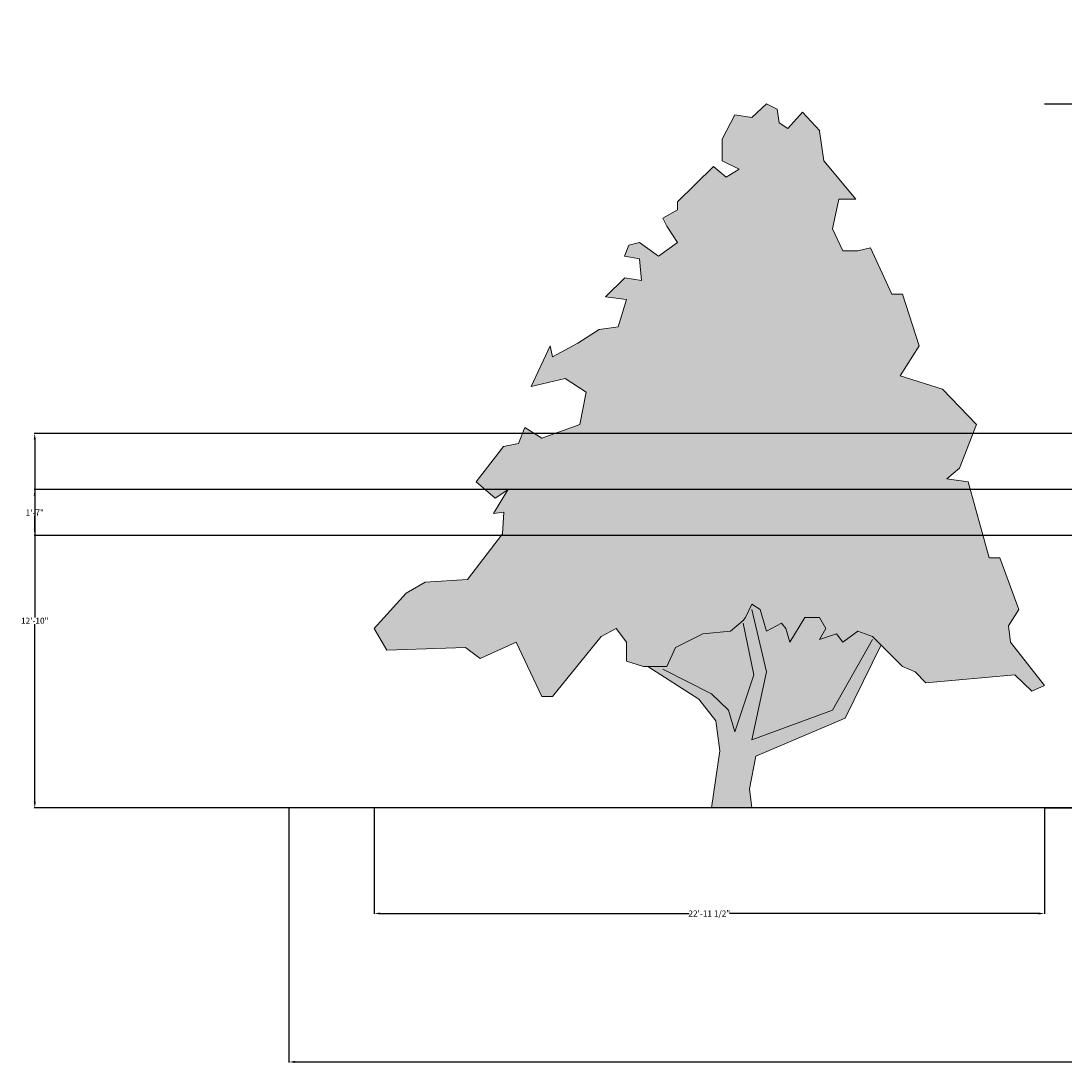
# Model space of a CAD drawing. Units: inches. Extents: x 481 to 2783, y 1975 to 3327.
# Tile 1 of 13: x 481 to 910, y 2015 to 2447. Entities that reach past the tile are written whole.
import ezdxf

# ---------------------------------------------------------------- set-up
doc = ezdxf.new("R2010")
doc.units = ezdxf.units.IN
doc.header["$MEASUREMENT"] = 0
for name, color, linetype, lineweight in [('A-ANNO-DIMS', 50, 'Continuous', 18), ('C-TOPO', 7, 'Continuous', 25), ('L-PLNT', 7, 'Continuous', 13)]:
    doc.layers.add(name, color=color, linetype=linetype, lineweight=lineweight)
doc.layers.add('L-PLNT-PATT', color=116, linetype='Continuous', lineweight=13, true_color=0x136734)
doc.layers.add('L-PLNT-TRNK-PATT', color=249, linetype='Continuous', lineweight=13, true_color=0x593132)
doc.styles.get("Standard").update_dxf_attribs({"font": 'arial.ttf'})
doc.dimstyles.get("Standard").update_dxf_attribs({"dimtxt": 2.5, "dimasz": 2.5, "dimexe": 0.18, "dimexo": 0.0625, "dimgap": 0.09, "dimtad": 0, "dimtih": 1, "dimtoh": 1, "dimzin": 0, "dimdsep": 46, "dimlunit": 3, "dimtxsty": 'Standard', "dimcen": 0.09, "dimadec": 0, "dimazin": 0, "dimtfac": 1, "dimtofl": 0, "dimtmove": 0, "dimatfit": 3, "dimfxl": 1, "dimtolj": 1, "dimtzin": 0, "dimarcsym": 0})

# ---------------------------------------------------------------- blocks, each defined once
blk = doc.blocks.new('Tree - type 3 evergreen elevation')
for points in [[(22.0124, 137.721), (18.5475, 141.5624), (15.5282, 138.2446), (13.8028, 139.3505), (13.3714, 142.1153), (11.2148, 143.2214), (8.1954, 140.4564), (4.7447, 141.0094), (2.1567, 136.0326), (2.1567, 131.6088), (5.6074, 129.9499), (3.0193, 128.2909), (0.4313, 130.5029), (-6.9015, 123.3141), (-6.9015, 121.6552), (-9.9208, 119.9963), (-9.0581, 118.3373), (-6.9015, 115.0195), (-10.7835, 112.2546), (-14.6656, 115.0195), (-16.8222, 114.4665), (-17.6849, 112.2546), (-14.6656, 111.7016), (-14.2342, 107.2778), (-17.6065, 107.8307), (-21.5669, 103.9599), (-17.2536, 103.4069), (-18.9789, 97.8771), (-22.8609, 97.3241), (-27.1743, 94.5593), (-32.3504, 91.7944), (-32.7817, 94.0063), (-36.6638, 85.7116), (-29.7624, 87.3705), (-25.449, 84.6056), (-26.743, 77.9699), (-34.507, 75.205), (-37.9578, 77.4169), (-39.2518, 74.099), (-42.2711, 73.5461), (-44.8592, 70.2282), (-47.8786, 66.3574), (-43.9965, 63.0395), (-41.4085, 64.6985), (-44.3346, 59.8898), (-42.2089, 60.1377), (-42.5159, 55.7849), (-49.6039, 46.4502), (-58.2307, 45.8972), (-62.1127, 43.6853), (-68.5828, 36.4966), (-65.9947, 32.0727), (-50.0352, 32.6257), (-47.0159, 30.4138), (-39.6831, 33.7317), (-34.507, 22.6721), (-32.3504, 22.6721), (-22.4296, 34.8376), (-19.4102, 36.4966), (-17.2536, 33.7317), (-17.2536, 29.8608), (-13.8028, 28.7549), (-9.0581, 28.7549), (-7.3328, 32.6257), (-1.7254, 35.3906), (3.8821, 35.9436), (6.4701, 38.1555), (6.9014, 38.7085), (8.1954, 41.4734), (9.9208, 40.3674), (11.2148, 35.9436), (14.2341, 37.6025), (15.0968, 36.4966), (15.9595, 33.7317), (18.9789, 38.7085), (21.9982, 38.7085), (23.2922, 36.4966), (21.9982, 34.2847), (25.4489, 35.3906), (26.743, 33.7317), (29.7623, 35.9436), (32.7817, 34.8376), (38.8204, 28.7549), (41.4084, 27.6489), (43.5651, 25.437), (61.6813, 27.0959), (65.132, 23.7781), (67.7201, 24.884), (60.8186, 33.7317), (60.3873, 37.0495), (62.544, 40.3674), (58.662, 50.874), (56.5053, 50.874), (52.1919, 66.3574), (47.8785, 66.9103), (50.4665, 69.1222), (53.9172, 77.9699), (47.0158, 85.1586), (38.3891, 87.9235), (42.2711, 94.0063)], [(42.2711, 94.0063), (38.8204, 104.5129), (36.6637, 104.5129), (32.3503, 113.9135), (29.7623, 113.3605), (26.743, 113.3605), (24.5862, 117.7844), (25.8802, 123.8671), (29.331, 123.8671), (22.8609, 131.6088), (21.9982, 137.6916)], [(8.1954, 40.3674), (11.2148, 27.6489), (8.1954, 13.8245), (24.5862, 19.9072), (32.7817, 34.2847)], [(-9.9208, 28.2019), (0, 23.2251), (3.4507, 19.9072), (4.7447, 15.4834), (8.6267, 27.0959), (6.4701, 37.6025)], [(34.5071, 33.1787), (27.1743, 18.2483), (9.0581, 10.5066), (7.7641, 3.8708), (8.1954, 0)], [(-12.9401, 28.7549), (-2.588, 22.1191), (0.8626, 17.6953), (1.7253, 11.6125), (0, 0)]]:
    blk.add_lwpolyline(points)
blk = doc.blocks.new('*D58')
at = {"layer": 'A-ANNO-DIMS', "color": 0, "lineweight": -2, "transparency": 16777216}
for p, q in [((901.81, 2412.41), (945.37, 2412.41)), ((945.19, 2409.91), (945.19, 2269)), ((945.19, 2125.32), (945.19, 2266.23)), ((901.81, 2122.82), (945.37, 2122.82))]:
    blk.add_line(p, q, dxfattribs=at)
at = {"layer": 'A-ANNO-DIMS', "color": 0, "transparency": 16777216}
for points in [[(944.77, 2409.91), (945.61, 2409.91), (945.19, 2412.41)], [(944.77, 2125.32), (945.61, 2125.32), (945.19, 2122.82)]]:
    blk.add_solid(points, dxfattribs=at)
at = {"layer": 'Defpoints', "color": 0, "transparency": 16777216}
for p in [(901.75, 2412.41), (945.19, 2412.41), (901.75, 2122.82)]:
    blk.add_point(p, dxfattribs=at)
at = {"layer": 'A-ANNO-DIMS', "color": 0, "transparency": 16777216, "insert": (945.19, 2267.62), "char_height": 2.5, "attachment_point": 5}
blk.add_mtext('\\A1;EVERGREEN 24\'-1 1/2"', dxfattribs=at)
blk = doc.blocks.new('*D59')
at = {"layer": 'A-ANNO-DIMS', "color": 0, "lineweight": -2, "transparency": 16777216}
for p, q in [((626.15, 2122.76), (626.15, 2079.2)), ((901.75, 2122.76), (901.75, 2079.2)), ((628.65, 2079.38), (755.66, 2079.38)), ((899.25, 2079.38), (772.24, 2079.38))]:
    blk.add_line(p, q, dxfattribs=at)
at = {"layer": 'A-ANNO-DIMS', "color": 0, "transparency": 16777216}
for points in [[(628.65, 2079.8), (628.65, 2078.97), (626.15, 2079.38)], [(899.25, 2079.8), (899.25, 2078.97), (901.75, 2079.38)]]:
    blk.add_solid(points, dxfattribs=at)
at = {"layer": 'Defpoints', "color": 0, "transparency": 16777216}
for p in [(626.15, 2122.82), (901.75, 2122.82), (901.75, 2079.38)]:
    blk.add_point(p, dxfattribs=at)
at = {"layer": 'A-ANNO-DIMS', "color": 0, "transparency": 16777216, "insert": (763.95, 2079.38), "char_height": 2.5, "attachment_point": 5}
blk.add_mtext('\\A1;22\'-11 1/2"', dxfattribs=at)
blk = doc.blocks.new('*D66')
at = {"layer": 'A-ANNO-DIMS', "color": 0, "lineweight": -2, "transparency": 16777216}
for p, q in [((591.06, 2122.76), (591.06, 2018.14)), ((2669.26, 2122.76), (2669.26, 2018.14)), ((593.56, 2018.32), (1624.92, 2018.32)), ((2666.76, 2018.32), (1635.4, 2018.32))]:
    blk.add_line(p, q, dxfattribs=at)
at = {"layer": 'A-ANNO-DIMS', "color": 0, "transparency": 16777216}
for points in [[(593.56, 2018.74), (593.56, 2017.9), (591.06, 2018.32)], [(2666.76, 2018.74), (2666.76, 2017.9), (2669.26, 2018.32)]]:
    blk.add_solid(points, dxfattribs=at)
at = {"layer": 'Defpoints', "color": 0, "transparency": 16777216}
for p in [(591.06, 2122.82), (2669.26, 2122.82), (2669.26, 2018.32)]:
    blk.add_point(p, dxfattribs=at)
at = {"layer": 'A-ANNO-DIMS', "color": 0, "transparency": 16777216, "insert": (1630.16, 2018.32), "char_height": 2.5, "attachment_point": 5}
blk.add_mtext('\\A1;173\'-2"', dxfattribs=at)
blk = doc.blocks.new('*D67')
at = {"layer": 'A-ANNO-DIMS', "color": 0, "lineweight": -2, "transparency": 16777216}
for p, q in [((591.06, 2122.76), (591.06, 2018.14)), ((1374.44, 2122.76), (1374.44, 2018.14)), ((593.56, 2018.32), (975.45, 2018.32)), ((1371.94, 2018.32), (990.05, 2018.32))]:
    blk.add_line(p, q, dxfattribs=at)
at = {"layer": 'A-ANNO-DIMS', "color": 0, "transparency": 16777216}
for points in [[(593.56, 2018.74), (593.56, 2017.9), (591.06, 2018.32)], [(1371.94, 2018.74), (1371.94, 2017.9), (1374.44, 2018.32)]]:
    blk.add_solid(points, dxfattribs=at)
at = {"layer": 'Defpoints', "color": 0, "transparency": 16777216}
for p in [(591.06, 2122.82), (1374.44, 2122.82), (1374.44, 2018.32)]:
    blk.add_point(p, dxfattribs=at)
at = {"layer": 'A-ANNO-DIMS', "color": 0, "transparency": 16777216, "insert": (982.75, 2018.32), "char_height": 2.5, "attachment_point": 5}
blk.add_mtext('\\A1;65\'-3 1/2"', dxfattribs=at)
blk = doc.blocks.new('*D69')
at = {"layer": 'A-ANNO-DIMS', "color": 0, "lineweight": -2, "transparency": 16777216}
for p, q in [((1374.38, 2276.82), (486.38, 2276.82)), ((486.56, 2274.32), (486.56, 2201.19)), ((486.56, 2125.32), (486.56, 2198.45)), ((1374.38, 2122.82), (486.38, 2122.82))]:
    blk.add_line(p, q, dxfattribs=at)
at = {"layer": 'A-ANNO-DIMS', "color": 0, "transparency": 16777216}
for points in [[(486.15, 2274.32), (486.98, 2274.32), (486.56, 2276.82)], [(486.15, 2125.32), (486.98, 2125.32), (486.56, 2122.82)]]:
    blk.add_solid(points, dxfattribs=at)
at = {"layer": 'Defpoints', "color": 0, "transparency": 16777216}
for p in [(486.56, 2276.82), (1374.44, 2276.82), (1374.44, 2122.82)]:
    blk.add_point(p, dxfattribs=at)
at = {"layer": 'A-ANNO-DIMS', "color": 0, "transparency": 16777216, "insert": (486.56, 2199.82), "char_height": 2.5, "attachment_point": 5}
blk.add_mtext('\\A1;12\'-10"', dxfattribs=at)
blk = doc.blocks.new('*D73')
at = {"layer": 'A-ANNO-DIMS', "color": 0, "lineweight": -2, "transparency": 16777216}
for p, q in [((1392.88, 2253.82), (486.38, 2253.82)), ((486.56, 2251.32), (486.56, 2245.67)), ((486.56, 2237.32), (486.56, 2242.98)), ((1392.88, 2234.82), (486.38, 2234.82))]:
    blk.add_line(p, q, dxfattribs=at)
at = {"layer": 'A-ANNO-DIMS', "color": 0, "transparency": 16777216}
for points in [[(486.15, 2251.32), (486.98, 2251.32), (486.56, 2253.82)], [(486.15, 2237.32), (486.98, 2237.32), (486.56, 2234.82)]]:
    blk.add_solid(points, dxfattribs=at)
at = {"layer": 'Defpoints', "color": 0, "transparency": 16777216}
for p in [(486.56, 2253.82), (1392.94, 2253.82), (1392.94, 2234.82)]:
    blk.add_point(p, dxfattribs=at)
at = {"layer": 'A-ANNO-DIMS', "color": 0, "transparency": 16777216, "insert": (486.56, 2244.32), "char_height": 2.5, "attachment_point": 5}
blk.add_mtext('\\A1;1\'-7"', dxfattribs=at)

msp = doc.modelspace()

# ---------------------------------------------------------------- hatches: boundary and pattern name
at = {"layer": 'L-PLNT-PATT'}
h = msp.add_hatch(color=256, dxfattribs=at)
h.set_gradient(color1=(88, 186, 72), color2=(19, 155, 72))
h.paths.add_polyline_path([(2073.399, 2314.279), (2090.767, 2317.288), (2085.135, 2318.49), (2094.991, 2323.306), (2089.828, 2324.508), (2100.155, 2326.915), (2106.727, 2331.73), (2098.278, 2329.324), (2087.483, 2331.128), (2078.563, 2335.339), (2086.542, 2335.339), (2088.89, 2344.968), (2096.401, 2353.393), (2097.339, 2361.817), (2097.807, 2364.826), (2093.114, 2358.808), (2083.726, 2352.791), (2065.42, 2355.8), (2056.503, 2366.631), (2060.727, 2368.438), (2049.462, 2371.446), (2057.441, 2377.462), (2047.583, 2375.055), (2049.93, 2379.269), (2046.644, 2380.471), (2057.909, 2384.684), (2070.584, 2386.489), (2051.807, 2390.702), (2043.828, 2399.729), (2043.36, 2402.736), (2048.992, 2405.745), (2054.155, 2405.745), (2039.603, 2411.763), (2031.624, 2421.994), (2025.25, 2446.511), (2019.075, 2422.889), (2009.519, 2414.722), (1993.59, 2409.276), (1987.217, 2401.106), (1993.59, 2403.829), (1999.96, 2402.468), (2003.146, 2392.939), (1995.712, 2382.046), (1985.093, 2375.239), (1981.906, 2372.517), (1990.404, 2373.878), (1989.34, 2371.156), (1974.473, 2361.624), (1955.358, 2353.456), (1940.49, 2342.566), (1935.182, 2334.396), (1940.49, 2337.119), (1950.049, 2339.841), (1955.358, 2337.119), (1959.605, 2337.119), (1967.481, 2340.003), (1976.598, 2337.119), (1984.031, 2337.119), (1979.784, 2330.312), (1987.217, 2330.312), (1980.845, 2320.783), (1953.235, 2305.807), (1952.172, 2297.639), (1940.49, 2282.662), (1915.005, 2271.772), (1900.138, 2267.686), (1895.89, 2262.241), (1904.385, 2258.157), (1906.508, 2260.879), (1918.191, 2262.241), (1924.562, 2254.073), (1941.554, 2256.796), (1946.863, 2264.963), (1964.916, 2255.434), (1957.483, 2255.434), (1954.296, 2251.35), (1967.039, 2245.903), (1963.855, 2232.29), (1952.172, 2217.313), (1933.057, 2214.591), (1924.562, 2199.614), (1922.439, 2205.062), (1913.942, 2196.892), (1899.074, 2194.169), (1885.27, 2194.169), (1874.651, 2200.976), (1875.712, 2192.808), (1882.084, 2188.724), (1884.207, 2184.64), (1894.827, 2186.001), (1887.393, 2173.748), (1901.199, 2176.47), (1901.199, 2165.58), (1910.758, 2171.025), (1921.375, 2172.386), (1918.191, 2165.58), (1919.253, 2158.773), (1926.686, 2158.773), (1944.738, 2164.218), (1951.11, 2171.025), (1953.235, 2158.773), (1964.916, 2153.326), (1967.039, 2157.412), (1976.598, 2161.496), (1981.906, 2157.412), (1986.156, 2149.242), (2001.024, 2158.773), (2004.208, 2149.242), (2020.139, 2158.773), (2023.325, 2151.965), (2057.305, 2143.797), (2046.687, 2150.603), (2064.738, 2146.519), (2057.305, 2151.965), (2072.172, 2153.326), (2084.917, 2149.242), (2096.598, 2150.603), (2083.856, 2157.412), (2113.591, 2157.412), (2135.892, 2151.965), (2128.458, 2160.135), (2130.581, 2166.941), (2145.448, 2154.689), (2162.438, 2153.326), (2185.803, 2161.496), (2180.492, 2165.58), (2170.935, 2164.218), (2170.935, 2169.664), (2163.502, 2169.664), (2163.502, 2177.831), (2157.129, 2177.831), (2150.759, 2187.363), (2148.634, 2181.918), (2142.262, 2183.279), (2133.767, 2191.447), (2122.086, 2191.447), (2112.527, 2191.447), (2097.66, 2199.614), (2122.086, 2215.952), (2142.262, 2215.952), (2136.953, 2226.845), (2152.882, 2232.29), (2163.502, 2230.929), (2159.254, 2241.819), (2144.387, 2239.096), (2123.147, 2241.819), (2115.713, 2251.35), (2109.341, 2248.625), (2105.093, 2258.157), (2095.537, 2255.434), (2084.917, 2264.963), (2098.723, 2271.772), (2123.147, 2274.495), (2128.458, 2286.746), (2137.368, 2296.744), (2125.033, 2304.65), (2124.563, 2310.066), (2117.522, 2304.65), (2100.155, 2302.845), (2083.726, 2306.457)])
h.paths.add_polyline_path([(726.446, 2320.727), (718.597, 2319.609), (709.875, 2314.018), (699.409, 2308.428), (698.537, 2312.9), (690.688, 2296.128), (704.642, 2299.483), (713.364, 2293.892), (710.747, 2280.475), (695.049, 2274.884), (688.071, 2279.357), (685.455, 2272.648), (679.35, 2271.53), (674.117, 2264.821), (668.011, 2256.995), (675.861, 2250.286), (681.094, 2253.64), (675.177, 2243.917), (679.476, 2244.418), (678.855, 2235.617), (664.523, 2216.742), (647.08, 2215.624), (639.23, 2211.152), (626.148, 2196.616), (631.381, 2187.671), (663.651, 2188.789), (669.756, 2184.317), (684.583, 2191.026), (695.049, 2168.663), (699.409, 2168.663), (719.469, 2193.262), (725.574, 2196.616), (729.935, 2191.026), (729.935, 2183.199), (736.912, 2180.963), (746.506, 2180.963), (749.995, 2188.789), (761.333, 2194.38), (772.671, 2195.498), (777.904, 2199.971), (778.776, 2201.089), (781.392, 2206.679), (784.881, 2204.443), (787.498, 2195.498), (793.603, 2198.852), (795.347, 2196.616), (797.091, 2191.026), (803.197, 2201.089), (809.302, 2201.089), (811.918, 2196.616), (809.302, 2192.144), (816.279, 2194.38), (818.895, 2191.026), (825, 2195.498), (831.106, 2193.262), (843.316, 2180.963), (848.549, 2178.726), (852.91, 2174.254), (889.54, 2177.608), (896.518, 2170.9), (901.751, 2173.136), (887.796, 2191.026), (886.924, 2197.734), (891.285, 2204.443), (883.435, 2225.687), (879.075, 2225.687), (870.353, 2256.995), (861.631, 2258.112), (866.864, 2262.585), (873.841, 2280.475), (859.887, 2295.01), (842.444, 2300.601), (850.293, 2312.9), (843.316, 2334.144), (838.955, 2334.144), (830.233, 2353.152), (825, 2352.034), (818.895, 2352.034), (814.534, 2360.979), (817.151, 2373.278), (824.128, 2373.278), (811.046, 2388.932), (809.286, 2401.34), (802.324, 2409.058), (796.219, 2402.35), (792.731, 2404.586), (791.858, 2410.176), (787.498, 2412.413), (781.392, 2406.822), (774.415, 2407.94), (769.182, 2397.877), (769.182, 2388.932), (776.16, 2385.578), (770.926, 2382.223), (765.694, 2386.696), (750.867, 2372.16), (750.867, 2368.806), (744.762, 2365.452), (746.506, 2362.097), (750.867, 2355.389), (743.017, 2349.798), (735.168, 2355.389), (730.807, 2354.271), (729.063, 2349.798), (735.168, 2348.68), (736.04, 2339.735), (729.221, 2340.853), (721.213, 2333.026), (729.935, 2331.908)])
at = {"layer": 'L-PLNT-TRNK-PATT'}
h = msp.add_hatch(color=256, dxfattribs=at)
h.paths.add_polyline_path([(2529.81, 2146.699), (2570.983, 2164.294), (2587.589, 2198.106), (2583.727, 2201.997), (2576.865, 2204.51), (2570.003, 2199.483), (2567.062, 2203.254), (2559.219, 2200.74), (2562.16, 2205.767), (2559.219, 2210.794), (2552.357, 2210.794), (2545.495, 2199.483), (2543.534, 2205.767), (2541.573, 2208.281), (2534.711, 2204.51), (2531.77, 2214.564), (2527.849, 2217.078), (2524.908, 2210.794), (2523.928, 2209.537), (2518.046, 2204.51), (2505.302, 2203.254), (2492.558, 2196.97), (2488.637, 2188.172), (2479.814, 2188.172), (2503.341, 2173.091), (2511.184, 2163.037), (2513.144, 2149.213), (2509.223, 2122.821), (2527.849, 2122.821), (2526.869, 2131.618)])
h.paths.add_polyline_path([(834.542, 2189.801), (831.106, 2193.262), (825, 2195.498), (818.895, 2191.026), (816.279, 2194.38), (809.302, 2192.144), (811.918, 2196.616), (809.302, 2201.089), (803.197, 2201.089), (797.091, 2191.026), (795.347, 2196.616), (793.603, 2198.852), (787.498, 2195.498), (784.881, 2204.443), (781.392, 2206.679), (778.776, 2201.089), (777.904, 2199.971), (772.671, 2195.498), (761.333, 2194.38), (749.995, 2188.789), (746.506, 2180.963), (738.657, 2180.963), (759.589, 2167.545), (766.566, 2158.6), (768.31, 2146.301), (764.821, 2122.821), (781.392, 2122.821), (780.52, 2130.647), (783.137, 2144.065), (819.768, 2159.718)])

# ---------------------------------------------------------------- linework, layer by layer
at = {"layer": 'C-TOPO'}
msp.add_line((1374.438, 2122.821), (591.063, 2122.821), dxfattribs=at)

# ---------------------------------------------------------------- block references
at = {"layer": 'L-PLNT', "xscale": 2.021988810055089, "yscale": 2.021988810055089, "zscale": 2.021988810055089}
msp.add_blockref('Tree - type 3 evergreen elevation', (764.821, 2122.821), dxfattribs=at)

# ---------------------------------------------------------------- dimensions: what is measured, and where the dimension line sits
at = {"layer": 'A-ANNO-DIMS'}
dim = msp.add_linear_dim(base=(945.19, 2412.413), p1=(901.751, 2122.821), p2=(901.751, 2412.413), angle=90, text='EVERGREEN <>', dimstyle='Standard', override={"dimdec": 1, "dimlfac": 1, "dimrnd": 0, "dimzin": 1, "dimdsep": 46, "dimlunit": 4, "dimfrac": 2}, dxfattribs=at)
dim.commit()
dim.dimension.update_dxf_attribs({"geometry": '*D58', "text_midpoint": (945.19, 2267.617)})
for base, p1, p2, picture, middle in [((486.563, 2276.821), (1374.438, 2122.821), (1374.438, 2276.821), '*D69', (486.563, 2199.821)), ((486.563, 2253.821), (1392.938, 2234.821), (1392.938, 2253.821), '*D73', (486.563, 2244.321))]:
    dim = msp.add_linear_dim(base=base, p1=p1, p2=p2, angle=90, dimstyle='Standard', override={"dimdec": 1, "dimlfac": 1, "dimrnd": 0, "dimzin": 1, "dimdsep": 46, "dimlunit": 4, "dimfrac": 2}, dxfattribs=at)
    dim.commit()
    dim.dimension.update_dxf_attribs({"geometry": picture, "text_midpoint": middle})
for base, p1, p2, picture, middle in [((2669.257, 2018.321), (591.063, 2122.821), (2669.257, 2122.821), '*D66', (1630.16, 2018.321)), ((1374.438, 2018.321), (591.063, 2122.821), (1374.438, 2122.821), '*D67', (982.75, 2018.321)), ((901.751, 2079.382), (626.148, 2122.821), (901.751, 2122.821), '*D59', (763.949, 2079.382))]:
    dim = msp.add_linear_dim(base=base, p1=p1, p2=p2, dimstyle='Standard', override={"dimdec": 1, "dimlfac": 1, "dimrnd": 0, "dimzin": 1, "dimdsep": 46, "dimlunit": 4, "dimfrac": 2}, dxfattribs=at)
    dim.commit()
    dim.dimension.update_dxf_attribs({"geometry": picture, "text_midpoint": middle})

doc.saveas('drawing.dxf')
